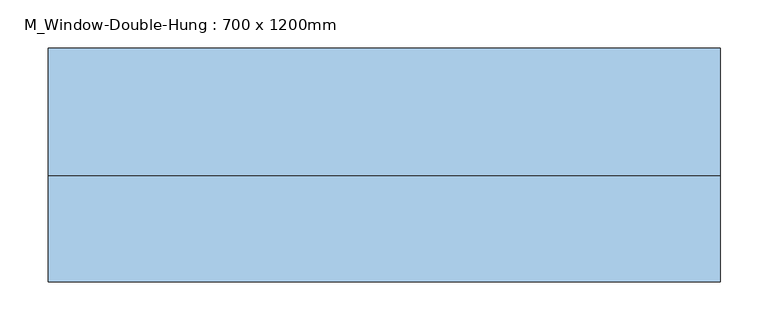
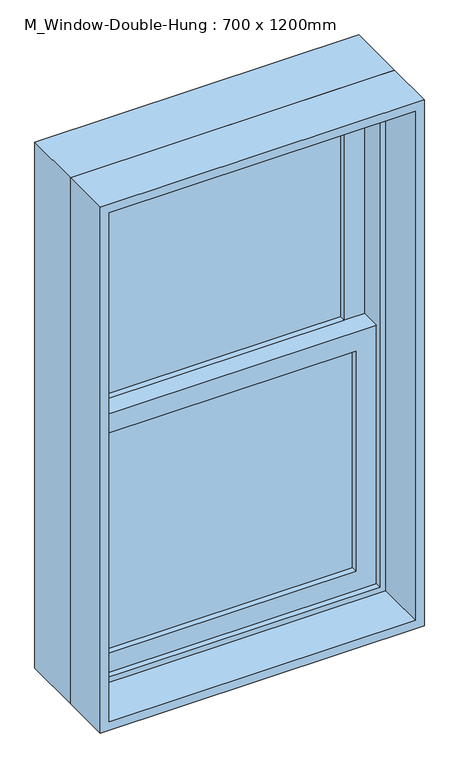
"""IFC4 building model written with IfcOpenShell, lengths in millimetres: window geometry, M_Window-Double-Hung : 700 x 1200mm."""

from ifc_helpers import new_model, si_unit, frame, origin, place, context, project, spatial, polyline, outline, extrude, source, transform, mapped, element, save


def m_window_double_hung_700_x_1200mm_9cb858e8(model_context):
    return source(origin(), model_context, "Body", "SweptSolid", [
        extrude(outline(polyline([(2114.4, 350.0), (2114.4, -350.0), (914.4, -350.0), (914.4, 350.0), (2114.4, 350.0)]), holes=[polyline([(2095.35, 330.95), (933.45, 330.95), (933.45, -330.95), (2095.35, -330.95), (2095.35, 330.95)])]), frame((0.0, -112.5, 0.0), z_axis=(0.0, 1.0, 0.0), x_axis=(0.0, 0.0, 1.0)), (0.0, 0.0, 1.0), 110.7),
        extrude(outline(polyline([(2114.4, -350.0), (914.4, -350.0), (914.4, 350.0), (2114.4, 350.0), (2114.4, -350.0)]), holes=[polyline([(2082.65, 318.25), (946.15, 318.25), (946.15, -318.25), (2082.65, -318.25), (2082.65, 318.25)])]), frame((0.0, -1.8, 0.0), z_axis=(0.0, 1.0, 0.0), x_axis=(0.0, 0.0, 1.0)), (0.0, 0.0, 1.0), 133.35),
        extrude(outline(polyline([(2082.65, -318.25), (1492.175, -318.25), (1492.175, 318.25), (2082.65, 318.25), (2082.65, -318.25)]), holes=[polyline([(2038.2, 273.8), (1536.625, 273.8), (1536.625, -273.8), (2038.2, -273.8), (2038.2, 273.8)])]), frame((0.0, 55.35, 0.0), z_axis=(0.0, 1.0, 0.0), x_axis=(0.0, 0.0, 1.0)), (0.0, 0.0, 1.0), 44.45),
        extrude(outline(polyline([(1536.625, -318.25), (946.15, -318.25), (946.15, 318.25), (1536.625, 318.25), (1536.625, -318.25)]), holes=[polyline([(1492.175, 273.8), (990.6, 273.8), (990.6, -273.8), (1492.175, -273.8), (1492.175, 273.8)])]), frame((0.0, 10.9, 0.0), z_axis=(0.0, 1.0, 0.0), x_axis=(0.0, 0.0, 1.0)), (0.0, 0.0, 1.0), 44.45),
        extrude(outline(polyline([(273.8, 87.1), (273.8, 80.75), (-273.8, 80.75), (-273.8, 87.1), (273.8, 87.1)])), frame((0.0, 0.0, 1536.625), z_axis=(0.0, 0.0, 1.0), x_axis=(1.0, 0.0, 0.0)), (0.0, 0.0, 1.0), 501.575),
        extrude(outline(polyline([(-273.8, 74.4), (273.8, 74.4), (273.8, 68.05), (-273.8, 68.05), (-273.8, 74.4)])), frame((0.0, 0.0, 1536.625), z_axis=(0.0, 0.0, 1.0), x_axis=(1.0, 0.0, 0.0)), (0.0, 0.0, 1.0), 501.575),
        extrude(outline(polyline([(273.8, 42.65), (273.8, 36.3), (-273.8, 36.3), (-273.8, 42.65), (273.8, 42.65)])), frame((0.0, 0.0, 990.6), z_axis=(0.0, 0.0, 1.0), x_axis=(1.0, 0.0, 0.0)), (0.0, 0.0, 1.0), 501.575),
        extrude(outline(polyline([(-273.8, 29.95), (273.8, 29.95), (273.8, 23.6), (-273.8, 23.6), (-273.8, 29.95)])), frame((0.0, 0.0, 990.6), z_axis=(0.0, 0.0, 1.0), x_axis=(1.0, 0.0, 0.0)), (0.0, 0.0, 1.0), 501.575),
    ])


if __name__ == "__main__":
    model = new_model("IFC4")
    model_context = context("Model", 3, world=origin())
    ifc_project = project(units=[si_unit("LENGTHUNIT", "METRE", prefix="MILLI")], contexts=[model_context])
    site = spatial("IfcSite", under=ifc_project)
    building = spatial("IfcBuilding", under=site)
    placement = place(None, origin())
    m_window_double_hung_700_x_1200mm_shape = m_window_double_hung_700_x_1200mm_9cb858e8(model_context)
    element("IfcWindow", 1, ObjectType="M_Window-Double-Hung : 700 x 1200mm", at=placement, inside=building, context=model_context, shape_type="MappedRepresentation", body=[
        mapped(m_window_double_hung_700_x_1200mm_shape, transform((0.0, 0.0, 0.0), x_axis=(1.0, 0.0, 0.0), y_axis=(0.0, 1.0, 0.0), z_axis=(0.0, 0.0, 1.0))),
    ])
    save(model, "model.ifc")

# Revit data of these elements
# Type "M_Window-Double-Hung : 700 x 1200mm"
#   Type Mark = "30"
#   Fire Rating = "0.5h"
#   Construction Type Id = "DG-DR"
#   Assembly Code = "B2020100"
#   Analytic Construction = "Double glazing - domestic"
#   Wall Thickness [instance default] = 150 mm
#   Window Inset [instance default] = 0 mm
#   Visual Light Transmittance = 0.81
#   Thermal Resistance (R) = 0.319569 (m²·K)/W
#   Solar Heat Gain Coefficient = 0.76
#   Muntin Width = 547.6 mm
#   Muntin Height = 501.575 mm
#   Interior Wall Closure [instance default] = 35.7 mm
#   Rough Width = 715 mm
#   Rough Height = 1215 mm
#   Frame Extension [instance default] = 31.75 mm
#   Exterior Wall Closure [instance default] = 12.7 mm
#   Extension Jamb [instance default] = 35.7 mm
#   Heat Transfer Coefficient (U) = 3.12929 W/(m²·K)
#   Height = 1200 mm
#   Width = 700 mm
#   Top Muntin Visibility = yes
#   Indicator Visibility [instance default] = yes
#   Extension Jamb Visibility [instance default] = yes
#   Interior Trim Visibility [instance default] = yes
#   Exterior Trim Visibility [instance default] = yes
#   Define Thermal Properties by = 1
#   Bottom Muntin Visibility = yes
#   Muntin Pattern = M_Muntin Pattern_2x2 : M_Muntin Pattern_2x2
#   Interior Trim Material = Wood - Stained
#   Interior Trim = M_Trim-Window-Interior-Flat : Picture Frame
#   Exterior Trim Material = Clad - White
#   Exterior Trim = M_Trim-Window-Exterior-Flat : with Sill
#   Glass Panel Material = Glass
#   Exterior Frame Material = Clad - White
#   Interior Frame Material = Wood - Stained
#   Wall Closure = (empty or 0)
# Element 1 (IfcWindow, "M_Window-Double-Hung : 700 x 1200mm")
#   Wall Thickness = 225 mm
#   Extension Jamb = 110.7 mm
#   Materials on its faces: "Wood - Stained", "Glass", "Clad - White"
# Materials
#   "Wood - Stained": class "Wood", colour RGB 173 132 96, transparency 0, Cost = 0
#   "Clad - White": class "Wood", colour RGB 245 245 243, transparency 0, Cost = 0
#   "Glass": class "Glass", colour RGB 245 245 243, transparency 1, Description = "Soda Lime Glass", Cost = 0
